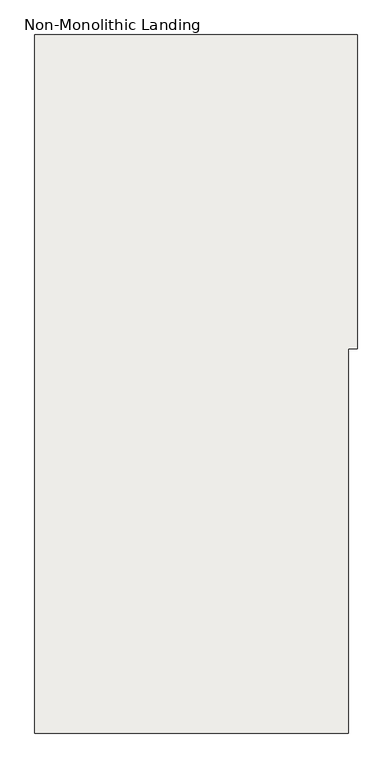
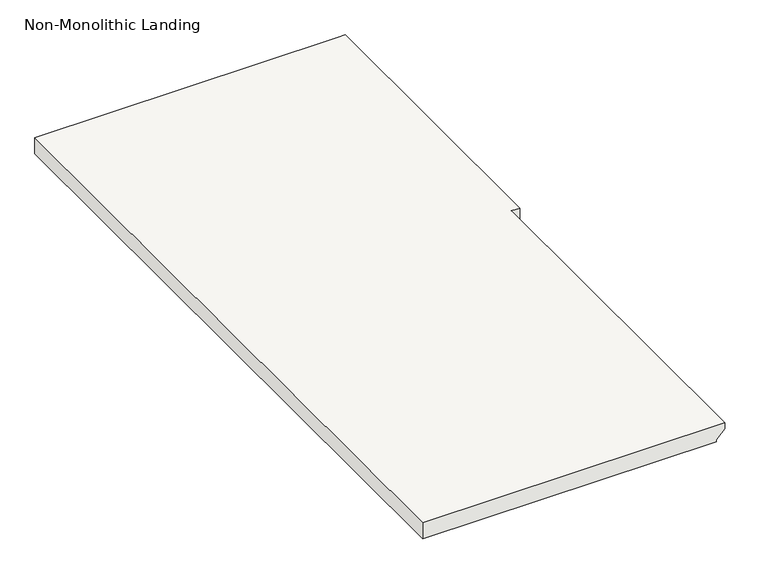
"""IFC4 building model written with IfcOpenShell, lengths in millimetres: slab geometry, Non-Monolithic Landing."""

from ifc_helpers import new_model, si_unit, origin, place, context, project, spatial, faceted_brep, source, transform, mapped, element, save


def non_monolithic_landing_2ab6d15e(model_context):
    return source(origin(), model_context, "Body", "Brep", [
        faceted_brep([(10553.9752377, 20886.8384539, 1936.75), (10528.5752377, 20886.8384539, 1911.35), (10528.5752377, 21801.2384539, 1911.35), (10553.9752377, 21801.2384539, 1936.75), (10553.9752377, 22006.2919009, 1955.8), (10579.3752377, 22006.2919009, 1955.8), (10579.3752377, 22920.6919009, 1955.8), (10553.9752377, 22920.6919009, 1955.8), (9639.5752377, 22920.6919009, 1955.8), (9639.5752377, 20886.8384539, 1955.8), (10553.9752377, 20886.8384539, 1955.8), (10528.5752377, 21801.2384539, 1905.0), (10528.5752377, 20886.8384539, 1905.0), (9639.5752377, 20886.8384539, 1905.0), (9639.5752377, 22920.6919009, 1905.0), (10553.9752377, 22920.6919009, 1905.0), (10579.3752377, 22920.6919009, 1905.0), (10579.3752377, 22006.2919009, 1905.0), (10553.9752377, 22006.2919009, 1905.0), (10553.9752377, 21801.2384539, 1905.0)], [[[0, 1, 2, 3]], [[4, 5, 6, 7, 8, 9, 10]], [[11, 12, 13, 14, 15, 16, 17, 18, 19]], [[12, 11, 2, 1]], [[11, 19, 3, 2]], [[4, 10, 0, 3, 19, 18]], [[5, 4, 18, 17]], [[6, 5, 17, 16]], [[7, 6, 16, 15]], [[8, 7, 15, 14]], [[9, 8, 14, 13]], [[10, 9, 13, 12, 1, 0]]]),
    ])


if __name__ == "__main__":
    model = new_model("IFC4")
    model_context = context("Model", 3, world=origin())
    ifc_project = project(units=[si_unit("LENGTHUNIT", "METRE", prefix="MILLI")], contexts=[model_context])
    site = spatial("IfcSite", under=ifc_project)
    building = spatial("IfcBuilding", under=site)
    placement = place(None, origin())
    non_monolithic_landing_shape = non_monolithic_landing_2ab6d15e(model_context)
    element("IfcSlab", 1, ObjectType="Non-Monolithic Landing", at=placement, inside=building, context=model_context, shape_type="MappedRepresentation", body=[
        mapped(non_monolithic_landing_shape, transform((0.0, 0.0, 0.0), x_axis=(1.0, 0.0, 0.0), y_axis=(0.0, 1.0, 0.0), z_axis=(0.0, 0.0, 1.0))),
    ])
    save(model, "model.ifc")
